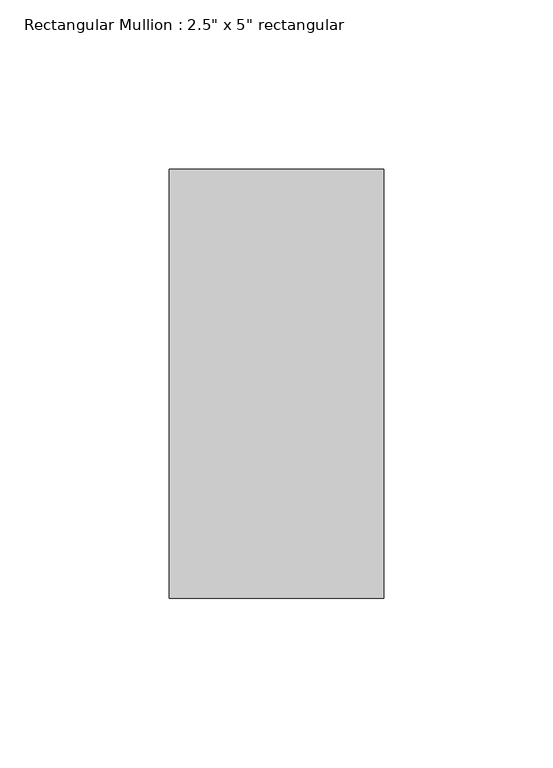
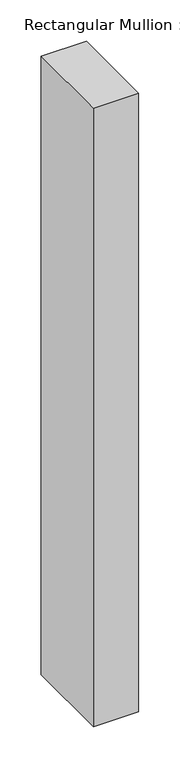
"""IFC4 building model written with IfcOpenShell, lengths in millimetres: member geometry."""

from ifc_helpers import new_model, si_unit, frame, origin, place, context, project, spatial, polyline, outline, extrude, source, transform, mapped, element, save


def member_2c52e315(model_context):
    return source(origin(), model_context, "Body", "SweptSolid", [
        extrude(outline(polyline([(0.0, 63.5), (0.0, -63.5), (-63.5, -63.5), (-63.5, 63.5), (0.0, 63.5)])), frame((0.0, 0.0, -915.6997825), z_axis=(0.0, 0.0, 1.0), x_axis=(1.0, 0.0, 0.0)), (0.0, 0.0, 1.0), 915.6997825),
    ])


if __name__ == "__main__":
    model = new_model("IFC4")
    model_context = context("Model", 3, world=origin())
    ifc_project = project(units=[si_unit("LENGTHUNIT", "METRE", prefix="MILLI")], contexts=[model_context])
    site = spatial("IfcSite", under=ifc_project)
    building = spatial("IfcBuilding", under=site)
    placement = place(None, origin())
    member_shape = member_2c52e315(model_context)
    element("IfcMember", 1, ObjectType="Rectangular Mullion : 2.5\" x 5\" rectangular", at=placement, inside=building, context=model_context, shape_type="MappedRepresentation", body=[
        mapped(member_shape, transform((0.0, 0.0, 0.0), x_axis=(1.0, 0.0, 0.0), y_axis=(0.0, 1.0, 0.0), z_axis=(0.0, 0.0, 1.0))),
    ])
    save(model, "model.ifc")

# Revit data of these elements
# Type "Rectangular Mullion : 2.5\" x 5\" rectangular"
#   built-in parameter 1007304 = 0.416667 (stored number, unit not read)
#   built-in parameter 1007301 = 0.104167 (stored number, unit not read)
#   built-in parameter 1007300 = 0.104167 (stored number, unit not read)
# Element 1 (IfcMember, "Rectangular Mullion : 2.5\" x 5\" rectangular")
#   Materials on its faces: "BLACK COLOUR"
# Materials
#   "BLACK COLOUR": class "Generic", colour RGB 120 120 120, transparency 0, Cost = 0
